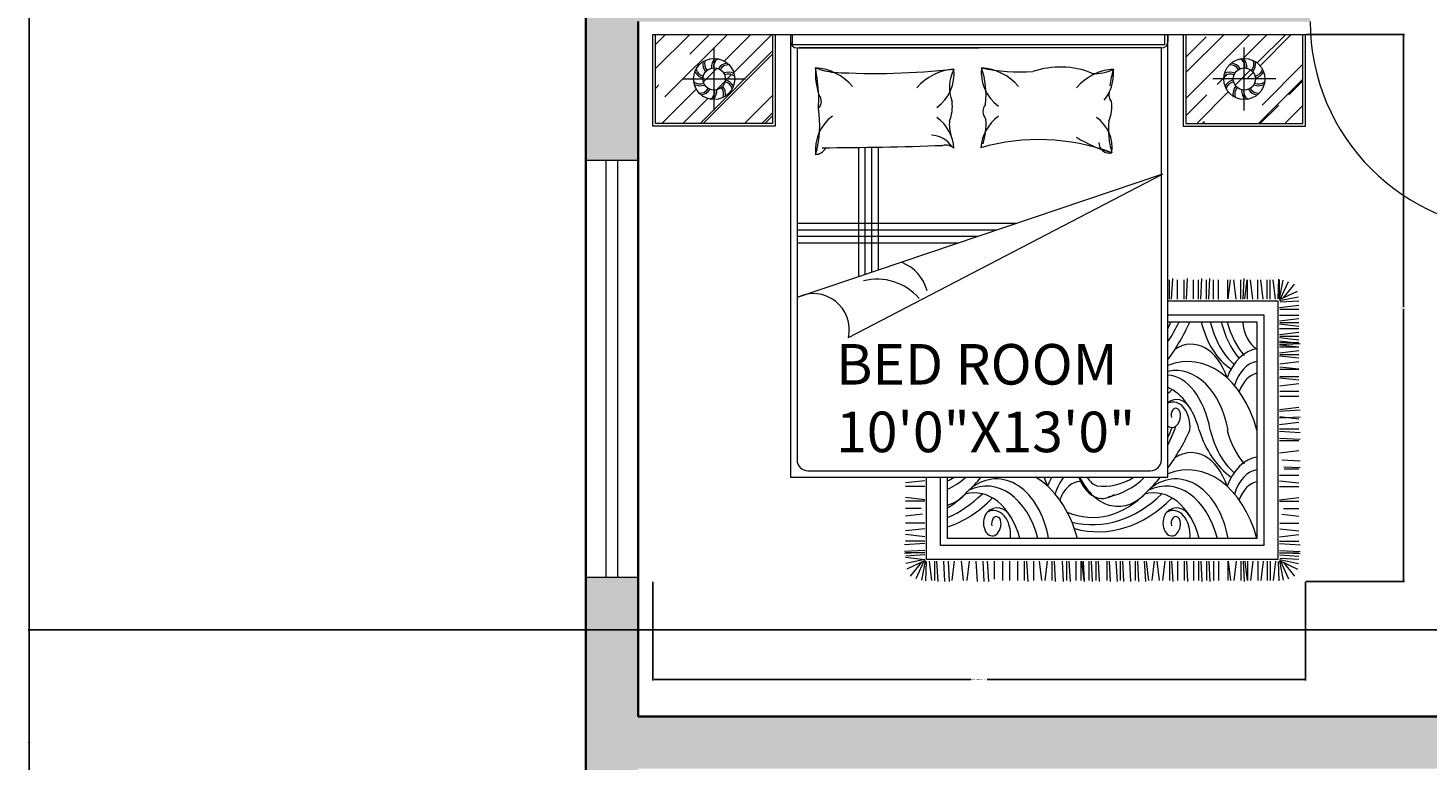
# Model space of a CAD drawing. Units: inches. Extents: x 2540 to 3167, y 3083 to 4007.
# Tile 9 of 15: x 2540 to 2782, y 3542 to 3669. Entities that reach past the tile are written whole.
import ezdxf

# ---------------------------------------------------------------- set-up
doc = ezdxf.new("R2010")
doc.units = ezdxf.units.IN
for name, color, linetype, lineweight in [('A-ANNO-DIMS', 2, 'Continuous', 18), ('A-AREA-IDEN', 7, 'Continuous', 18), ('A-DOOR', 4, 'Continuous', 18), ('A-FURN', 8, 'Continuous', 13), ('A-GLAZ', 4, 'Continuous', 18)]:
    doc.layers.add(name, color=color, linetype=linetype, lineweight=lineweight)
doc.layers.add('A-WALL', color=143, linetype='Continuous', lineweight=35, true_color=0x7aafdf)
doc.layers.add('A-WALL-PATT', color=143, linetype='Continuous', lineweight=13, true_color=0x7aafdf)
doc.styles.get("Standard").update_dxf_attribs({"font": 'arial.ttf'})
doc.dimstyles.get("Standard").update_dxf_attribs({"dimtxt": 0.18, "dimasz": 0.18, "dimexe": 0.18, "dimexo": 0.0625, "dimgap": 0.09, "dimtad": 0, "dimtih": 1, "dimtoh": 1, "dimdec": 4, "dimzin": 0, "dimdsep": 46, "dimtxsty": 'Standard', "dimcen": 0.09, "dimadec": 0, "dimazin": 0, "dimtfac": 1, "dimtdec": 4, "dimtofl": 0, "dimtmove": 0, "dimatfit": 3, "dimfxl": 1, "dimtolj": 1, "dimtzin": 0, "dimarcsym": 0})

# ---------------------------------------------------------------- blocks, each defined once
blk = doc.blocks.new('A$C64B41DC1')
for p, q in [((0, 2.5079), (2.9903, 2.5079)), ((0, 2.0879), (0, 2.5079)), ((0.012, 2.4618), (0.0581, 2.5079)), ((0.012, 2.3515), (0.1684, 2.5079)), ((0.012, 2.0999), (0.012, 2.5079)), ((0.0543, 2.2213), (0.3409, 2.5079)), ((0.1689, 2.4179), (0.2589, 2.5079)), ((0.3265, 2.386), (0.4484, 2.5079)), ((0.3699, 2.3332), (0.5445, 2.5079)), ((0.548, 2.5079), (0.548, 2.0999)), ((0.56, 2.5079), (0.56, 2.0879)), ((0.6301, 2.5079), (0.6301, 0.4779)), ((0.6401, 2.461), (0.6401, 2.5079)), ((0.6401, 2.5079), (2.344, 2.5079)), ((2.344, 2.5079), (2.3601, 2.5079)), ((2.344, 2.5079), (2.344, 2.461)), ((2.3601, 2.5079), (2.3601, 2.4761)), ((2.3601, 0.4779), (2.3601, 2.5079)), ((2.4303, 2.5079), (2.4303, 2.0879)), ((2.4423, 2.5079), (2.4423, 2.0999)), ((2.4423, 2.3333), (2.6169, 2.5079)), ((2.4423, 2.2145), (2.7357, 2.5079)), ((2.705, 2.398), (2.8149, 2.5079)), ((2.7691, 2.3772), (2.8998, 2.5079)), ((2.7819, 2.3646), (2.9252, 2.5079)), ((2.9783, 2.0999), (2.9783, 2.5079)), ((2.9903, 2.0879), (2.9903, 2.5079)), ((0.2804, 2.1597), (0.2804, 2.4481)), ((2.344, 2.461), (0.6401, 2.461)), ((0.6601, 2.4461), (1.4951, 2.4461)), ((0.6601, 2.4461), (0.6601, 0.5579)), ((1.4951, 2.4461), (0.6697, 2.4461)), ((2.3301, 2.4461), (1.4951, 2.4461)), ((2.3301, 0.5579), (2.3301, 2.4461)), ((2.4423, 2.404), (2.5354, 2.4971)), ((2.7099, 2.1597), (2.7099, 2.4481)), ((0.2157, 2.0999), (0.548, 2.4322)), ((0.2299, 2.0999), (0.548, 2.418)), ((0.2311, 2.2906), (0.2937, 2.3532)), ((0.3405, 2.3039), (0.3605, 2.3238)), ((2.6158, 2.3088), (2.6313, 2.3243)), ((2.6674, 2.2756), (2.7382, 2.3464)), ((2.7249, 2.3076), (2.7512, 2.3339)), ((2.7914, 2.1846), (2.9783, 2.3715)), ((0.012, 2.261), (0.0275, 2.2765)), ((0.0404, 2.0999), (0.1982, 2.2578)), ((0.1362, 2.3039), (0.4246, 2.3039)), ((0.2905, 2.2539), (0.3304, 2.2938)), ((2.8541, 2.3039), (2.5657, 2.3039)), ((2.5849, 2.2779), (2.6158, 2.3088)), ((2.7746, 2.0999), (2.9783, 2.3036)), ((2.9144, 2.2312), (2.9783, 2.2951)), ((0.1365, 2.0999), (0.251, 2.2144)), ((0.4194, 2.0999), (0.548, 2.2285)), ((2.4423, 2.1353), (2.5382, 2.2312)), ((2.4918, 2.0999), (2.6366, 2.2447)), ((2.7831, 2.0999), (2.8678, 2.1846)), ((2.8962, 2.0999), (2.9783, 2.182)), ((0.4986, 2.0999), (0.548, 2.1493)), ((0.5127, 2.0999), (0.548, 2.1352)), ((0.56, 2.0879), (0, 2.0879)), ((0.548, 2.0999), (0.012, 2.0999)), ((2.4303, 2.0879), (2.9903, 2.0879)), ((2.4423, 2.0999), (2.9783, 2.0999)), ((2.5172, 2.0999), (2.5269, 2.1096)), ((0.9415, 1.9902), (0.9415, 1.3975)), ((0.9715, 1.9906), (0.9715, 1.4076)), ((1.0015, 1.991), (1.0015, 1.4177)), ((1.0315, 1.9916), (1.0315, 1.4279)), ((2.3349, 1.8678), (0.6613, 1.3029)), ((0.8956, 1.1191), (2.3349, 1.8678)), ((1.6636, 1.6412), (0.6601, 1.6412)), ((1.5748, 1.6112), (0.6601, 1.6112)), ((2.3665, 1.295), (2.3665, 1.3839)), ((2.377, 1.295), (2.3822, 1.3891)), ((2.4032, 1.295), (2.4032, 1.3839)), ((2.4346, 1.295), (2.4346, 1.3839)), ((2.4451, 1.295), (2.4503, 1.3891)), ((2.4774, 1.2957), (2.4774, 1.3837)), ((2.5, 1.295), (2.5, 1.3839)), ((2.5105, 1.295), (2.5157, 1.3891)), ((2.5367, 1.295), (2.5367, 1.3839)), ((2.5471, 1.295), (2.5524, 1.3891)), ((2.5681, 1.295), (2.5681, 1.3839)), ((2.5918, 1.295), (2.5918, 1.3839)), ((2.6346, 1.2957), (2.6346, 1.3837)), ((2.6362, 1.2957), (2.6467, 1.3839)), ((2.6729, 1.295), (2.6624, 1.3839)), ((2.6938, 1.295), (2.6938, 1.3839)), ((2.7043, 1.295), (2.7095, 1.3891)), ((2.7127, 1.2957), (2.7232, 1.3839)), ((2.7253, 1.295), (2.7253, 1.3839)), ((2.7494, 1.295), (2.7389, 1.3839)), ((2.7718, 1.295), (2.7718, 1.3839)), ((2.7959, 1.295), (2.7854, 1.3839)), ((2.8146, 1.2957), (2.8146, 1.3837)), ((2.8146, 1.2957), (2.8146, 1.3837)), ((2.8282, 1.295), (2.8282, 1.3839)), ((2.8282, 1.295), (2.8282, 1.3839)), ((2.8523, 1.295), (2.8418, 1.3839)), ((2.8523, 1.295), (2.8418, 1.3839)), ((2.8653, 1.2966), (2.8688, 1.3861)), ((2.8711, 1.2957), (2.8711, 1.3837)), ((2.8711, 1.2957), (2.8875, 1.3822)), ((2.8765, 1.2958), (2.9132, 1.3758)), ((2.8893, 1.3011), (2.9394, 1.3636)), ((2.3601, 1.2873), (2.8639, 1.2873)), ((2.8639, 1.2873), (2.8639, 0.1018)), ((2.8713, 1.2927), (2.954, 1.3315)), ((2.8717, 1.2884), (2.9588, 1.3058)), ((2.8744, 1.2817), (2.9603, 1.2869)), ((2.3601, 1.2233), (2.7999, 1.2233)), ((2.7999, 1.2233), (2.7999, 0.1658)), ((2.8716, 1.2565), (2.9605, 1.2669)), ((2.8716, 1.2212), (2.9605, 1.2212)), ((2.8723, 1.2489), (2.9603, 1.2489)), ((2.3601, 1.1913), (2.7679, 1.1912)), ((2.7679, 1.1912), (2.7679, 0.1978)), ((2.8716, 1.1947), (2.9605, 1.2052)), ((2.8716, 1.181), (2.9605, 1.1705)), ((2.8716, 1.1595), (2.9605, 1.1595)), ((2.8723, 1.1872), (2.9603, 1.1872)), ((2.8716, 1.133), (2.9605, 1.1435)), ((2.8716, 1.1193), (2.9605, 1.1088)), ((2.8716, 1.1035), (2.9605, 1.093)), ((2.8716, 1.0965), (2.9605, 1.0965)), ((2.8716, 1.086), (2.9657, 1.0913)), ((2.8723, 1.1255), (2.9603, 1.1255)), ((2.8716, 1.0756), (2.9605, 1.0756)), ((2.8716, 1.0491), (2.9605, 1.0596)), ((2.8716, 1.0354), (2.9605, 1.0249)), ((2.8723, 1.0858), (2.9605, 1.0753)), ((2.8723, 1.0416), (2.9603, 1.0416)), ((2.8723, 0.9987), (2.9605, 1.0092)), ((2.8723, 0.985), (2.9605, 0.9745)), ((2.8723, 0.9735), (2.9603, 0.9735)), ((2.8716, 0.9346), (2.9605, 0.9241)), ((2.8723, 0.9408), (2.9603, 0.9408)), ((2.8723, 0.8979), (2.9605, 0.9084)), ((2.8723, 0.8726), (2.9603, 0.8726)), ((2.8723, 0.8505), (2.9603, 0.8505)), ((2.8716, 0.7885), (2.9605, 0.799)), ((2.8716, 0.7818), (2.9657, 0.787)), ((2.8716, 0.7503), (2.9657, 0.7556)), ((2.8716, 0.7204), (2.9605, 0.7309)), ((2.8723, 0.7571), (2.9605, 0.7466)), ((2.8716, 0.6995), (2.9605, 0.6995)), ((2.8716, 0.689), (2.9657, 0.6838)), ((2.8716, 0.6576), (2.9657, 0.6523)), ((2.8716, 0.6471), (2.9605, 0.6471)), ((2.8716, 0.5903), (2.9605, 0.6007)), ((2.882, 0.5582), (2.9657, 0.5536)), ((2.8909, 0.5263), (2.9657, 0.5222)), ((2.8928, 0.5169), (2.9605, 0.5169)), ((0.6301, 0.4779), (2.3601, 0.4779)), ((0.7101, 0.5079), (2.2801, 0.5079)), ((1.2465, 0.4625), (1.1576, 0.452)), ((1.2542, 0.1018), (1.2542, 0.4779)), ((1.3182, 0.1658), (1.3182, 0.4779)), ((1.3502, 0.1978), (1.3502, 0.4779)), ((2.8716, 0.4877), (2.9603, 0.4877)), ((2.8716, 0.4625), (2.9605, 0.452)), ((1.2465, 0.3746), (1.1576, 0.3851)), ((1.2465, 0.4365), (1.1577, 0.4365)), ((2.8716, 0.4365), (2.9603, 0.4365)), ((2.8716, 0.3746), (2.9605, 0.3851)), ((1.2465, 0.3684), (1.1577, 0.3684)), ((1.2285, 0.3357), (1.1577, 0.3357)), ((2.8716, 0.3684), (2.9603, 0.3684)), ((2.8896, 0.3357), (2.9603, 0.3357)), ((1.2355, 0.3092), (1.1576, 0.3)), ((1.2457, 0.2676), (1.1577, 0.2676)), ((2.8723, 0.2676), (2.9603, 0.2676)), ((2.8826, 0.3092), (2.9605, 0.3)), ((1.2457, 0.2423), (1.1576, 0.2319)), ((1.2465, 0.2057), (1.1576, 0.2161)), ((2.7679, 0.1978), (1.3502, 0.1978)), ((2.8716, 0.2057), (2.9605, 0.2161)), ((2.8723, 0.2423), (2.9605, 0.2319)), ((1.2465, 0.1742), (1.1524, 0.169)), ((1.2465, 0.1428), (1.1524, 0.1376)), ((1.2465, 0.1334), (1.1524, 0.1281)), ((1.2465, 0.1847), (1.1576, 0.1847)), ((1.2465, 0.1323), (1.1576, 0.1323)), ((1.2465, 0.1323), (1.1576, 0.1323)), ((2.7999, 0.1658), (1.3182, 0.1658)), ((2.8716, 0.1847), (2.9605, 0.1847)), ((2.8716, 0.1742), (2.9657, 0.169)), ((2.8716, 0.1428), (2.9657, 0.1376)), ((2.8716, 0.1334), (2.9657, 0.1281)), ((2.8716, 0.1323), (2.9605, 0.1323)), ((1.2465, 0.1), (1.1576, 0.1105)), ((1.2465, 0.1229), (1.1588, 0.1168)), ((1.2464, 0.1007), (1.1592, 0.0833)), ((1.2468, 0.0964), (1.1641, 0.0576)), ((1.2288, 0.088), (1.1787, 0.0255)), ((1.2415, 0.0933), (1.2049, 0.0133)), ((1.247, 0.0934), (1.2306, 0.0069)), ((1.2527, 0.0925), (1.2493, 0.003)), ((2.8639, 0.1018), (1.2542, 0.1018)), ((1.2658, 0.0941), (1.2762, 0.0052)), ((1.2899, 0.0941), (1.2899, 0.0052)), ((1.2999, 0.0941), (1.3051, 0)), ((1.3313, 0.0941), (1.3365, 0)), ((1.3523, 0.0941), (1.3575, 0)), ((1.3804, 0.0941), (1.3699, 0.0052)), ((1.4119, 0.0934), (1.4223, 0.0052)), ((1.4485, 0.0941), (1.438, 0.0052)), ((1.48, 0.0941), (1.4852, 0)), ((1.5114, 0.0941), (1.5166, 0)), ((1.5323, 0.0941), (1.5376, 0)), ((1.5638, 0.0941), (1.5638, 0.0105)), ((1.6021, 0.0941), (1.6021, 0.0052)), ((1.6336, 0.0941), (1.6336, 0.0052)), ((1.6702, 0.0941), (1.6702, 0.0052)), ((1.7017, 0.0941), (1.7017, 0.0052)), ((1.7122, 0.0941), (1.7174, 0)), ((1.7445, 0.0934), (1.7445, 0.0054)), ((1.7698, 0.0934), (1.7803, 0.0052)), ((1.8065, 0.0941), (1.796, 0.0052)), ((1.8274, 0.0941), (1.8274, 0.0052)), ((1.8379, 0.0941), (1.8431, 0)), ((1.8746, 0.0941), (1.8798, 0)), ((1.8955, 0.0941), (1.8955, 0.0052)), ((1.906, 0.0941), (1.9113, 0)), ((1.9384, 0.0934), (1.9384, 0.0054)), ((1.9609, 0.0941), (1.9609, 0.0052)), ((1.9636, 0.0934), (1.9741, 0.0052)), ((1.9714, 0.0941), (1.9766, 0)), ((1.9976, 0.0941), (1.9976, 0.0052)), ((2.0081, 0.0941), (2.0133, 0)), ((2.029, 0.0941), (2.029, 0.0052)), ((2.0395, 0.0941), (2.0447, 0)), ((2.0797, 0.0941), (2.0797, 0.0052)), ((2.0902, 0.0941), (2.0954, 0)), ((2.1216, 0.0941), (2.1269, 0)), ((2.1412, 0.0941), (2.1412, 0.0052)), ((2.1517, 0.0941), (2.1569, 0)), ((2.1831, 0.0941), (2.1884, 0)), ((2.2093, 0.0941), (2.2093, 0.0052)), ((2.2198, 0.0941), (2.225, 0)), ((2.2512, 0.0941), (2.2565, 0)), ((2.2603, 0.0934), (2.2707, 0.0052)), ((2.2969, 0.0941), (2.2864, 0.0052)), ((2.3089, 0.0934), (2.3193, 0.0052)), ((2.3455, 0.0941), (2.3351, 0.0052)), ((2.3665, 0.0941), (2.3665, 0.0052)), ((2.377, 0.0941), (2.3822, 0)), ((2.4032, 0.0941), (2.4032, 0.0052)), ((2.4346, 0.0941), (2.4346, 0.0052)), ((2.4451, 0.0941), (2.4503, 0)), ((2.4774, 0.0934), (2.4774, 0.0054)), ((2.5, 0.0941), (2.5, 0.0052)), ((2.5105, 0.0941), (2.5157, 0)), ((2.5367, 0.0941), (2.5367, 0.0052)), ((2.5471, 0.0941), (2.5524, 0)), ((2.5681, 0.0941), (2.5681, 0.0052)), ((2.5918, 0.0941), (2.5918, 0.0052)), ((2.6346, 0.0934), (2.6346, 0.0054)), ((2.6362, 0.0934), (2.6467, 0.0052)), ((2.6729, 0.0941), (2.6624, 0.0052)), ((2.6938, 0.0941), (2.6938, 0.0052)), ((2.7043, 0.0941), (2.7095, 0)), ((2.7127, 0.0934), (2.7232, 0.0052)), ((2.7253, 0.0941), (2.7253, 0.0052)), ((2.7494, 0.0941), (2.7389, 0.0052)), ((2.7718, 0.0941), (2.7718, 0.0052)), ((2.7959, 0.0941), (2.7854, 0.0052)), ((2.8146, 0.0934), (2.8146, 0.0054)), ((2.8282, 0.0941), (2.8282, 0.0052)), ((2.8523, 0.0941), (2.8418, 0.0052)), ((2.8653, 0.0925), (2.8688, 0.003)), ((2.8711, 0.0934), (2.8875, 0.0069)), ((2.8713, 0.0964), (2.954, 0.0576)), ((2.8716, 0.1229), (2.9593, 0.1168)), ((2.8717, 0.1007), (2.9588, 0.0833)), ((2.8744, 0.1074), (2.9603, 0.1022)), ((2.8765, 0.0933), (2.9132, 0.0133)), ((2.8893, 0.088), (2.9394, 0.0255))]:
    blk.add_line(p, q)
at = {"ltscale": 10}
for p, q in [((1.4859, 1.5812), (0.6601, 1.5812)), ((1.397, 1.5512), (0.6601, 1.5512))]:
    blk.add_line(p, q, dxfattribs=at)
for centre, radius in [((0.2804, 2.3039), 0.0942), ((2.7099, 2.3039), 0.0942), ((0.2804, 2.3039), 0.051), ((2.7099, 2.3039), 0.051)]:
    blk.add_circle(centre, radius)
for centre, radius, start, end in [((0.6601, 2.4761), 0.03, 180, 270), ((2.3301, 2.4761), 0.03, 270, 0), ((0.2887, 2.3745), 0.0605, 172.17003, 218.48975), ((0.2828, 2.3731), 0.0462, 160.30017, 220.53802), ((0.3286, 2.3561), 0.0605, 136.17003, 182.48975), ((0.3231, 2.3585), 0.0462, 124.30017, 184.53802), ((0.3501, 2.3178), 0.0605, 100.17003, 146.48975), ((2.6402, 2.3178), 0.0605, 33.51025, 79.82997), ((2.6672, 2.3585), 0.0462, 355.46198, 55.69983), ((2.6617, 2.3561), 0.0605, 357.51025, 43.82997), ((2.7075, 2.3731), 0.0462, 319.46198, 19.69983), ((2.7016, 2.3745), 0.0605, 321.51025, 7.82997), ((0.2457, 2.3659), 0.0605, 208.17003, 254.48975), ((0.2417, 2.3614), 0.0462, 196.30017, 256.53802), ((0.347, 2.323), 0.0462, 88.30017, 148.53802), ((0.3449, 2.2742), 0.0605, 64.17003, 110.48975), ((0.3455, 2.2802), 0.0462, 52.30017, 112.53802), ((1.0526, 2.3302), 0.3085, 175.30484, 198.69419), ((-0.8702, 2.0941), 1.6364, 4.80985, 9.18918), ((0.8579, 2.6278), 0.2948, 247.51785, 264.26696), ((0.728, 2.111), 0.245, 40.4189, 85.9871), ((1.0164, 5.7096), 3.3803, 266.81337, 276.16021), ((1.3963, 2.1044), 0.245, 94.0129, 139.5811), ((1.1858, 2.3288), 0.1943, 306.5711, 5.88998), ((1.5348, 2.2652), 0.1767, 151.77364, 201.69827), ((1.6986, 2.3355), 0.1943, 174.11002, 233.4289), ((1.1481, 2.2311), 0.3783, 353.49469, 19.18669), ((1.6871, 3.192), 0.8561, 257.74383, 273.62843), ((1.4882, 2.111), 0.245, 40.4189, 85.9871), ((1.8674, 1.9709), 0.3878, 68.20259, 108.9817), ((2.1269, 2.1044), 0.245, 94.0129, 139.5811), ((2.0342, 2.4856), 0.1563, 261.59582, 298.90918), ((1.9165, 2.3288), 0.1943, 333.73715, 5.88998), ((2.6058, 2.2028), 0.517, 163.60457, 172.3273), ((2.6448, 2.2802), 0.0462, 67.46198, 127.69983), ((2.6454, 2.2742), 0.0605, 69.51025, 115.82997), ((2.6433, 2.323), 0.0462, 31.46198, 91.69983), ((2.7486, 2.3614), 0.0462, 283.46198, 343.69983), ((2.7446, 2.3659), 0.0605, 285.51025, 331.82997), ((0.2153, 2.3276), 0.0462, 232.30017, 292.53802), ((0.2158, 2.3336), 0.0605, 244.17003, 290.48975), ((0.2138, 2.2848), 0.0462, 268.30017, 328.53802), ((0.2107, 2.29), 0.0605, 280.17003, 326.48975), ((0.2377, 2.2493), 0.0462, 304.30017, 4.53802), ((0.2322, 2.2517), 0.0605, 316.17003, 2.48975), ((0.2779, 2.2347), 0.0462, 340.30017, 40.53802), ((0.272, 2.2333), 0.0605, 352.17003, 38.48975), ((0.3191, 2.2464), 0.0462, 16.30017, 76.53802), ((0.3151, 2.2419), 0.0605, 28.17003, 74.48975), ((2.6752, 2.2419), 0.0605, 105.51025, 151.82997), ((2.6712, 2.2464), 0.0462, 103.46198, 163.69983), ((2.7182, 2.2333), 0.0605, 141.51025, 187.82997), ((2.7123, 2.2347), 0.0462, 139.46198, 199.69983), ((2.7581, 2.2517), 0.0605, 177.51025, 223.82997), ((2.7526, 2.2493), 0.0462, 175.46198, 235.69983), ((2.7796, 2.29), 0.0605, 213.51025, 259.82997), ((2.7765, 2.2848), 0.0462, 211.46198, 271.69983), ((2.7744, 2.3336), 0.0605, 249.51025, 295.82997), ((2.775, 2.3276), 0.0462, 247.46198, 307.69983), ((0.7274, 2.2013), 0.0446, 314.4736, 42.17134), ((-1.6008, 2.277), 2.3618, 357.39054, 358.88764), ((1.204, 2.1778), 0.1681, 337.01697, 7.53676), ((1.5671, 2.1546), 0.0547, 142.08329, 220.902), ((1.9165, 2.3288), 0.1943, 320.94042, 333.73715), ((2.1347, 2.2313), 0.0459, 165.35061, 223.26844), ((1.9346, 2.1778), 0.1681, 337.01697, 7.53676), ((0.9385, 1.978), 0.1943, 126.5711, 185.88998), ((0.2688, 2.0945), 0.4956, 344.0243, 8.70709), ((1.1858, 1.9714), 0.1943, 4.31813, 53.4289), ((1.7059, 1.9714), 0.204, 127.11975, 175.09005), ((1.1965, 2.0983), 0.3299, 343.79543, 3.55541), ((1.9394, 1.991), 0.1651, 351.26213, 55.75721), ((1.5415, 2.0969), 0.1834, 175.22328, 196.23004), ((2.4617, 2.0719), 0.3745, 173.82958, 196.4356), ((0.7246, 18.8439), 16.8552, 270.17399, 272.05214), ((1.2687, 1.9248), 0.1223, 33.62799, 86.47438), ((1.3401, 1.9404), 0.0603, 49.09906, 101.37023), ((1.7676, 1.0629), 0.9631, 69.65065, 105.96307), ((2.2748, 2.5795), 0.6373, 238.34989, 254.31375), ((2.0911, 2.0123), 0.0478, 179.77267, 283.80184), ((0.7417, 2.0149), 0.057, 273.47085, 328.54118), ((0.728, 2.2025), 0.245, 274.0129, 278.34166), ((1.0747, 1.2871), 0.1871, 14.1863, 69.12121), ((1.0274, 1.1334), 0.2527, 40.62904, 104.37123), ((0.7347, 1.1553), 0.1649, 347.31088, 116.44537), ((0.7101, 0.5579), 0.05, 180, 270), ((2.2801, 0.5579), 0.05, 270, 0)]:
    blk.add_arc(centre, radius, start, end)
for centre, major_axis, ratio, start_param, end_param in [((1.9938, 1.6262), (0, -0.7531), 0.68, 0.797284, 0.954936), ((2.0643, 1.466), (0, -0.5322), 0.68, 7.239912, 7.311536), ((1.9052, 1.7397), (0, -0.9842), 0.68, 0.74745, 0.979724), ((2.7455, 1.3081), (0, 0.3614), 0.68, 1.900046, 2.742661), ((2.7868, 1.3081), (0, 0.3614), 0.68, 1.900046, 2.614747), ((2.8372, 1.3081), (0, 0.3614), 0.68, 1.900046, 2.479658), ((2.8607, 1.3211), (0, 0.3614), 0.68, 1.938265, 2.479658), ((2.8057, 1.2079), (0, -0.1524), 0.68, 4.821745, 5.895886), ((2.4665, 0.8216), (0, -0.2664), 0.68, 2.006169, 3.565187), ((2.4513, 0.5069), (0, 0.502), 0.68, 5.095327, 6.553458), ((2.7862, 0.8069), (0, -0.2615), 0.68, 3.244645, 4.205018), ((2.396, 0.6032), (0, 0.3641), 0.68, -1.3172, 0.145284), ((2.7784, 0.8289), (0, -0.1802), 0.68, 3.227058, 4.318474), ((2.3507, 0.5642), (0.0073, 0.3819), 0.56205, -1.21172, -0.009991), ((2.7821, 0.7971), (0, -0.1589), 0.68, 3.272942, 4.229533), ((2.2964, 0.5771), (0, -0.3263), 0.68, 1.938944, 2.850232), ((2.0403, 1.6015), (0, -0.8763), 0.68, 6.849801, 6.887077), ((2.4005, 0.7132), (0, -0.1214), 0.68, 2.284368, 3.652258), ((2.3834, 0.7081), (0, 0.1147), 0.68, 4.593909, 6.585576), ((2.3961, 0.7628), (0, -0.0317), 0.68, 1.462497, 5.046281), ((2.3774, 0.7653), (0, -0.0593), 0.68, 5.841311, 7.755362), ((1.9938, 1.1295), (-0.0678, 0.7439), 0.610498, 3.917146, 4.063997), ((2.0643, 0.9693), (0, -0.5322), 0.68, 7.239912, 7.336618), ((1.9052, 1.243), (0, -0.9842), 0.68, 0.74745, 0.979724), ((2.7455, 0.8114), (-0.0599, 0.3735), 0.695517, 1.775813, 2.548612), ((2.7868, 0.8114), (0, 0.3614), 0.68, 1.900046, 2.614747), ((2.8607, 0.8243), (0, 0.3614), 0.68, 1.938265, 2.479658), ((2.4665, 0.3249), (0, -0.2664), 0.68, 2.006169, 3.565187), ((2.4513, 0.0102), (0, 0.502), 0.68, 5.095327, 6.553458), ((2.7862, 0.3102), (0, -0.2615), 0.68, 3.244645, 4.205018), ((1.242, 0.9693), (0, -0.5322), 0.68, 6.586764, 6.677612), ((1.1714, 1.1295), (-0.1157, 0.7241), 0.59432, 3.291697, 3.50733), ((1.0828, 1.243), (0, -0.9842), 0.68, 0.565948, 0.680366), ((1.5283, 0.0674), (0, -0.3703), 0.68, 1.930561, 3.464283), ((1.5736, 0.1065), (0, 0.3641), 0.68, -1.3172, 0.476403), ((1.6289, 0.0102), (0, 0.502), 0.68, 6.655152, 6.661293), ((1.6289, 0.0102), (0, 0.502), 0.68, 5.095327, 5.911219), ((1.6442, 0.3249), (0, -0.2664), 0.68, 2.006169, 2.182797), ((1.9638, 0.3102), (0, -0.2615), 0.68, 4.015924, 4.205018), ((1.956, 0.3322), (0, -0.1802), 0.68, 3.770744, 4.318474), ((1.9597, 0.3004), (0, -0.1589), 0.68, 3.14258, 4.229533), ((2.0606, 0.5616), (0, -0.1803), 0.68, 5.194792, 5.929328), ((2.0606, 0.5616), (0, -0.1803), 0.68, 5.194792, 6.723255), ((2.1315, 0.6603), (0, -0.3155), 0.68, 5.328638, 6.949396), ((2.0549, 0.5656), (0, -0.1303), 0.68, 5.450951, 6.054641), ((2.0643, 0.9693), (0, -0.5322), 0.68, 6.20013, 6.677612), ((1.9938, 1.1295), (-0.0678, 0.7439), 0.610498, 3.199135, 3.592282), ((1.9052, 1.243), (0, -0.9842), 0.68, 0.565948, 0.680366), ((2.3507, 0.0674), (0, -0.3703), 0.68, 1.930561, 3.464283), ((2.396, 0.1065), (0, 0.3641), 0.68, -1.3172, 0.476403), ((2.4513, 0.0102), (0, 0.502), 0.68, 6.655152, 6.661293), ((2.7784, 0.3322), (0, -0.1802), 0.68, 3.227058, 4.318474), ((2.7821, 0.3004), (0, -0.1589), 0.68, 3.272942, 4.229533), ((1.1933, 0.9181), (0, -0.624), 0.68, 0.378672, 0.625379), ((1.3091, 0.6603), (0, -0.3155), 0.68, 6.475719, 6.949396), ((1.1911, 1.1066), (0, 0.8458), 0.68, 3.421828, 3.728616), ((1.474, 0.0804), (0, -0.3263), 0.68, 1.938944, 3.339184), ((2.0157, 0.9181), (0, -0.624), 0.68, -0.280078, 0.625379), ((2.0135, 1.1066), (0, 0.8458), 0.68, 2.978727, 3.728616), ((2.2964, 0.0804), (0, -0.3263), 0.68, 1.938944, 3.339184), ((1.2179, 1.1047), (0, -0.8763), 0.68, 6.507006, 6.887077), ((1.5781, 0.2165), (0, -0.1214), 0.68, 2.284368, 3.726131), ((1.561, 0.2114), (0, 0.1147), 0.68, 4.593909, 6.647252), ((2.0403, 1.1047), (0, -0.8763), 0.68, 6.099302, 6.887077), ((2.4005, 0.2165), (0, -0.1214), 0.68, 2.284368, 3.726131), ((2.3834, 0.2114), (0, 0.1147), 0.68, 4.593909, 6.647252), ((1.555, 0.2685), (0, -0.0593), 0.68, 3.732151, 7.755362), ((1.5737, 0.2661), (0, -0.0317), 0.68, 1.462497, 5.046281), ((2.3774, 0.2685), (0, -0.0593), 0.68, 3.732151, 7.755362), ((2.3961, 0.2661), (0, -0.0317), 0.68, 1.462497, 5.046281)]:
    blk.add_ellipse(centre, major_axis=major_axis, ratio=ratio, start_param=start_param, end_param=end_param)
blk = doc.blocks.new('DOOR-SWING-36IN')
for p, q in [((36, 0), (0, 0)), ((36, 1), (0.01, 1)), ((36, 1), (36, 0))]:
    blk.add_line(p, q)
blk.add_arc((36, 0), 36, 90, 180)
blk = doc.blocks.new('WIN-72IN')
for p, q in [((9, 72), (0, 72)), ((3.5, 0), (3.5, 72)), ((5.5, 0), (5.5, 72)), ((9, 0), (0, 0))]:
    blk.add_line(p, q)
blk = doc.blocks.new('*D31')
at = {"layer": 'A-ANNO-DIMS', "color": 0, "lineweight": -2, "transparency": 16777216}
for p, q in [((2648.08, 3572.96), (2648.08, 3555.95)), ((2760.71, 3572.96), (2760.71, 3555.95)), ((2648.26, 3556.13), (2703.01, 3556.13)), ((2760.53, 3556.13), (2705.78, 3556.13))]:
    blk.add_line(p, q, dxfattribs=at)
at = {"layer": 'A-ANNO-DIMS', "color": 0, "transparency": 16777216}
for points in [[(2648.26, 3556.16), (2648.26, 3556.1), (2648.08, 3556.13)], [(2760.53, 3556.16), (2760.53, 3556.1), (2760.71, 3556.13)]]:
    blk.add_solid(points, dxfattribs=at)
at = {"layer": 'Defpoints', "color": 0, "transparency": 16777216}
for p in [(2648.08, 3573.02), (2760.71, 3573.02), (2760.71, 3556.13)]:
    blk.add_point(p, dxfattribs=at)
at = {"layer": 'A-ANNO-DIMS', "color": 0, "transparency": 16777216, "insert": (2704.4, 3556.13), "char_height": 0.18, "attachment_point": 5}
blk.add_mtext('\\A1;BED GROUP 113 TYP.', dxfattribs=at)
blk = doc.blocks.new('*D32')
at = {"layer": 'A-ANNO-DIMS', "color": 0, "lineweight": -2, "transparency": 16777216}
for p, q in [((2760.77, 3667.48), (2777.79, 3667.48)), ((2777.61, 3667.3), (2777.61, 3620.43)), ((2777.61, 3573.2), (2777.61, 3620.07)), ((2760.77, 3573.02), (2777.79, 3573.02))]:
    blk.add_line(p, q, dxfattribs=at)
at = {"layer": 'A-ANNO-DIMS', "color": 0, "transparency": 16777216}
for points in [[(2777.58, 3667.3), (2777.64, 3667.3), (2777.61, 3667.48)], [(2777.58, 3573.2), (2777.64, 3573.2), (2777.61, 3573.02)]]:
    blk.add_solid(points, dxfattribs=at)
at = {"layer": 'Defpoints', "color": 0, "transparency": 16777216}
for p in [(2760.71, 3667.48), (2777.61, 3667.48), (2760.71, 3573.02)]:
    blk.add_point(p, dxfattribs=at)
at = {"layer": 'A-ANNO-DIMS', "color": 0, "transparency": 16777216, "insert": (2777.61, 3620.25), "char_height": 0.18, "attachment_point": 5}
blk.add_mtext('\\A1;94 TYP.', dxfattribs=at)
blk = doc.blocks.new('*D44')
at = {"layer": 'A-ANNO-DIMS', "color": 0, "lineweight": -2, "transparency": 16777216}
for p, q in [((2771.45, 3964.71), (2540.23, 3964.71)), ((2540.41, 3964.53), (2540.41, 3545.4)), ((2540.41, 3125.89), (2540.41, 3545.03)), ((2810.45, 3125.71), (2540.23, 3125.71))]:
    blk.add_line(p, q, dxfattribs=at)
at = {"layer": 'A-ANNO-DIMS', "color": 0, "transparency": 16777216}
for points in [[(2540.38, 3964.53), (2540.44, 3964.53), (2540.41, 3964.71)], [(2540.38, 3125.89), (2540.44, 3125.89), (2540.41, 3125.71)]]:
    blk.add_solid(points, dxfattribs=at)
at = {"layer": 'Defpoints', "color": 0, "transparency": 16777216}
for p in [(2540.41, 3964.71), (2771.51, 3964.71), (2810.51, 3125.71)]:
    blk.add_point(p, dxfattribs=at)
at = {"layer": 'A-ANNO-DIMS', "color": 0, "transparency": 16777216, "insert": (2540.41, 3545.21), "char_height": 0.18, "attachment_point": 5}
blk.add_mtext('\\A1;839', dxfattribs=at)
blk = doc.blocks.new('*D57')
at = {"layer": 'A-ANNO-DIMS', "color": 0, "lineweight": -2, "transparency": 16777216}
for p, q in [((2810.45, 3564.71), (2540.23, 3564.71)), ((2540.41, 3564.53), (2540.41, 3539.4)), ((2540.41, 3513.89), (2540.41, 3539.03)), ((2810.45, 3513.71), (2540.23, 3513.71))]:
    blk.add_line(p, q, dxfattribs=at)
at = {"layer": 'A-ANNO-DIMS', "color": 0, "transparency": 16777216}
for points in [[(2540.38, 3564.53), (2540.44, 3564.53), (2540.41, 3564.71)], [(2540.38, 3513.89), (2540.44, 3513.89), (2540.41, 3513.71)]]:
    blk.add_solid(points, dxfattribs=at)
at = {"layer": 'Defpoints', "color": 0, "transparency": 16777216}
for p in [(2810.51, 3564.71), (2540.41, 3513.71), (2810.51, 3513.71)]:
    blk.add_point(p, dxfattribs=at)
at = {"layer": 'A-ANNO-DIMS', "color": 0, "transparency": 16777216, "insert": (2540.41, 3539.21), "char_height": 0.18, "attachment_point": 5}
blk.add_mtext('\\A1;51', dxfattribs=at)

msp = doc.modelspace()

# ---------------------------------------------------------------- hatches: boundary and pattern name
at = {"layer": 'A-WALL-PATT'}
h = msp.add_hatch(color=256, dxfattribs=at)
h.dxf.hatch_style = 1
h.paths.add_polyline_path([(2805.51, 3803.71), (2800.51, 3803.71), (2800.51, 3799.71), (2621.51, 3799.71), (2621.51, 3823.71), (2612.51, 3823.71), (2612.51, 3794.71), (2636.51, 3794.71), (2636.51, 3782.71), (2645.51, 3782.71), (2645.51, 3794.71), (2805.51, 3794.71)])
h.paths.add_polyline_path([(2810.51, 3564.71), (2868.51, 3564.71), (2868.51, 3627.71), (2872.51, 3627.71), (2872.51, 3636.71), (2864.51, 3636.71), (2864.51, 3674.71), (2797.51, 3674.71), (2797.51, 3669.71), (2801.51, 3669.71), (2801.51, 3628.63), (2806.51, 3628.63), (2806.51, 3669.71), (2859.51, 3669.71), (2859.51, 3573.71), (2806.51, 3573.71), (2806.51, 3598.63), (2801.51, 3598.63), (2801.51, 3549.71), (2645.51, 3549.71), (2645.51, 3573.71), (2636.51, 3573.71), (2636.51, 3516.71), (2645.51, 3516.71), (2645.51, 3540.71), (2801.51, 3540.71), (2801.51, 3504.71), (2801.51, 3500.71), (2806.51, 3500.71), (2806.51, 3504.71), (2859.51, 3504.71), (2859.51, 3420.71), (2806.51, 3420.71), (2806.51, 3470.71), (2801.51, 3470.71), (2801.51, 3420.71), (2797.51, 3420.71), (2797.51, 3415.71), (2864.51, 3415.71), (2864.51, 3453.71), (2868.51, 3453.71), (2868.51, 3513.71), (2810.51, 3513.71)])
h.paths.add_polyline_path([(2645.51, 3415.71), (2761.51, 3415.71), (2761.51, 3420.71), (2645.51, 3420.71), (2645.51, 3444.71), (2636.51, 3444.71), (2636.51, 3403.71), (2645.51, 3403.71)])
h.paths.add_polyline_path([(2645.51, 3307.71), (2636.51, 3307.71), (2636.51, 3295.71), (2612.51, 3295.71), (2612.51, 3149.71), (2645.51, 3149.71), (2645.51, 3158.71), (2621.51, 3158.71), (2621.51, 3290.71), (2801.51, 3290.71), (2801.51, 3286.71), (2806.51, 3286.71), (2806.51, 3295.71), (2645.51, 3295.71)])
h.paths.add_polyline_path([(2762.01, 3158.71), (2746.51, 3158.71), (2746.51, 3240.71), (2750.51, 3240.71), (2750.51, 3245.71), (2741.51, 3245.71), (2741.51, 3158.71), (2717.51, 3158.71), (2717.51, 3149.71), (2762.01, 3149.71)], flags=17)
h.paths.add_polyline_path([(2810.51, 3173.71), (2822.51, 3173.71), (2822.51, 3182.71), (2806.51, 3182.71), (2806.51, 3250.71), (2801.51, 3250.71), (2801.51, 3245.71), (2780.51, 3245.71), (2780.51, 3240.71), (2801.51, 3240.71), (2801.51, 3158.71), (2786.01, 3158.71), (2786.01, 3149.71), (2810.51, 3149.71)])
h.paths.add_polyline_path([(2931.51, 3290.71), (2935.51, 3290.71), (2935.51, 3295.71), (2926.51, 3295.71), (2926.51, 3182.71), (2910.51, 3182.71), (2910.51, 3173.71), (2922.51, 3173.71), (2922.51, 3149.71), (2987.51, 3149.71), (2987.51, 3158.71), (2931.51, 3158.71)])
h.paths.add_polyline_path([(3124.51, 3295.71), (3086.51, 3295.71), (3018.51, 3295.71), (3018.51, 3290.71), (3115.51, 3290.71), (3115.51, 3158.71), (3059.51, 3158.71), (3059.51, 3149.71), (3124.51, 3149.71)])
h.paths.add_polyline_path([(2988.51, 3295.71), (2984.51, 3295.71), (2984.51, 3349.71), (3086.51, 3349.71), (3086.51, 3320.71), (3124.51, 3320.71), (3124.51, 3354.71), (3071.51, 3354.71), (3071.51, 3358.71), (3062.51, 3358.71), (3062.51, 3354.71), (2979.51, 3354.71), (2979.51, 3295.71), (2971.51, 3295.71), (2971.51, 3290.71), (2988.51, 3290.71)])
h.paths.add_polyline_path([(3095.51, 3325.71), (3095.51, 3349.71), (3119.51, 3349.71), (3119.51, 3325.71)], flags=16)
h.paths.add_polyline_path([(3124.51, 3462.71), (3071.51, 3462.71), (3071.51, 3627.71), (3124.51, 3627.71), (3124.51, 3693.71), (3095.51, 3693.71), (3095.51, 3702.71), (3086.51, 3702.71), (3086.51, 3684.71), (3086.51, 3636.71), (2930.51, 3636.71), (2930.51, 3768.71), (2934.51, 3768.71), (2934.51, 3773.71), (2930.51, 3773.71), (2925.51, 3773.71), (2925.51, 3730.71), (2864.51, 3730.71), (2864.51, 3760.71), (2859.51, 3760.71), (2859.51, 3725.71), (2925.51, 3725.71), (2925.51, 3636.71), (2908.51, 3636.71), (2908.51, 3627.71), (3062.51, 3627.71), (3062.51, 3543.71), (2930.51, 3543.71), (2930.51, 3534.71), (2993.51, 3534.71), (2993.51, 3516.71), (3002.51, 3516.71), (3002.51, 3534.71), (3062.51, 3534.71), (3062.51, 3462.71), (3002.51, 3462.71), (3002.51, 3480.71), (2993.51, 3480.71), (2993.51, 3462.71), (2916.51, 3462.71), (2916.51, 3453.71), (2926.51, 3453.71), (2926.51, 3361.71), (2859.51, 3361.71), (2859.51, 3338.71), (2864.51, 3338.71), (2864.51, 3356.71), (2926.51, 3356.71), (2926.51, 3338.71), (2931.51, 3338.71), (2931.51, 3453.71), (3062.51, 3453.71), (3062.51, 3448.21), (3071.51, 3448.21), (3071.51, 3453.71), (3124.51, 3453.71)])
h = msp.add_hatch(color=256, dxfattribs=at)
h.dxf.hatch_style = 1
h.paths.add_polyline_path([(3095.51, 3788.71), (3086.51, 3788.71), (3086.51, 3773.71), (3015.51, 3773.71), (3015.51, 3768.71), (3086.51, 3768.71), (3086.51, 3750.71), (3095.51, 3750.71)])
h.paths.add_polyline_path([(2645.51, 3669.71), (2761.51, 3669.71), (2761.51, 3674.71), (2645.51, 3674.71), (2645.51, 3686.71), (2636.51, 3686.71), (2636.51, 3645.71), (2645.51, 3645.71)])

# ---------------------------------------------------------------- linework, layer by layer
at = {"layer": 'A-WALL'}
for p, q in [((2636.51, 3686.71), (2636.51, 3403.71)), ((2645.51, 3669.71), (2645.51, 3549.71)), ((2645.51, 3549.71), (2801.51, 3549.71))]:
    msp.add_line(p, q, dxfattribs=at)

# ---------------------------------------------------------------- block references
at = {"layer": 'A-DOOR', "rotation": 89.99999999999872}
msp.add_blockref('DOOR-SWING-36IN', (2797.51, 3633.71), dxfattribs=at)
at = {"layer": 'A-FURN', "xscale": 37.66426153275995, "yscale": 37.66426153275995, "zscale": 37.66426153275995}
msp.add_blockref('A$C64B41DC1', (2648.08, 3573.02), dxfattribs=at)
at = {"layer": 'A-GLAZ'}
msp.add_blockref('WIN-72IN', (2636.51, 3573.71), dxfattribs=at)

# ---------------------------------------------------------------- texts
at = {"layer": 'A-AREA-IDEN', "insert": (2679.69, 3614.03), "char_height": 7, "attachment_point": 1}
msp.add_mtext_dynamic_manual_height_columns('BED ROOM\\P10\'0"X13\'0"', width=75.6369, gutter_width=12.5, heights=[0], dxfattribs=at)

# ---------------------------------------------------------------- dimensions: what is measured, and where the dimension line sits
at = {"layer": 'A-ANNO-DIMS'}
for base, p1, p2, picture, middle in [((2540.41, 3964.71), (2810.51, 3125.71), (2771.51, 3964.71), '*D44', (2540.41, 3545.21)), ((2540.41, 3513.71), (2810.51, 3564.71), (2810.51, 3513.71), '*D57', (2540.41, 3539.21))]:
    dim = msp.add_linear_dim(base=base, p1=p1, p2=p2, angle=90, dimstyle='Standard', override={"dimdec": 0, "dimlfac": 1, "dimrnd": 0, "dimzin": 0, "dimdsep": 46, "dimlunit": 2}, dxfattribs=at)
    dim.commit()
    dim.dimension.update_dxf_attribs({"geometry": picture, "text_midpoint": middle})
dim = msp.add_linear_dim(base=(2777.61, 3667.48), p1=(2760.71, 3573.02), p2=(2760.71, 3667.48), angle=90, text='<> TYP.', dimstyle='Standard', override={"dimdec": 0, "dimlfac": 1, "dimrnd": 0, "dimzin": 0, "dimdsep": 46, "dimlunit": 2}, dxfattribs=at)
dim.commit()
dim.dimension.update_dxf_attribs({"geometry": '*D32', "text_midpoint": (2777.61, 3620.25)})
dim = msp.add_linear_dim(base=(2760.71, 3556.13), p1=(2648.08, 3573.02), p2=(2760.71, 3573.02), text='BED GROUP <> TYP.', dimstyle='Standard', override={"dimdec": 0, "dimlfac": 1, "dimrnd": 0, "dimzin": 0, "dimdsep": 46, "dimlunit": 2}, dxfattribs=at)
dim.commit()
dim.dimension.update_dxf_attribs({"geometry": '*D31', "text_midpoint": (2704.4, 3556.13)})

doc.saveas('drawing.dxf')
